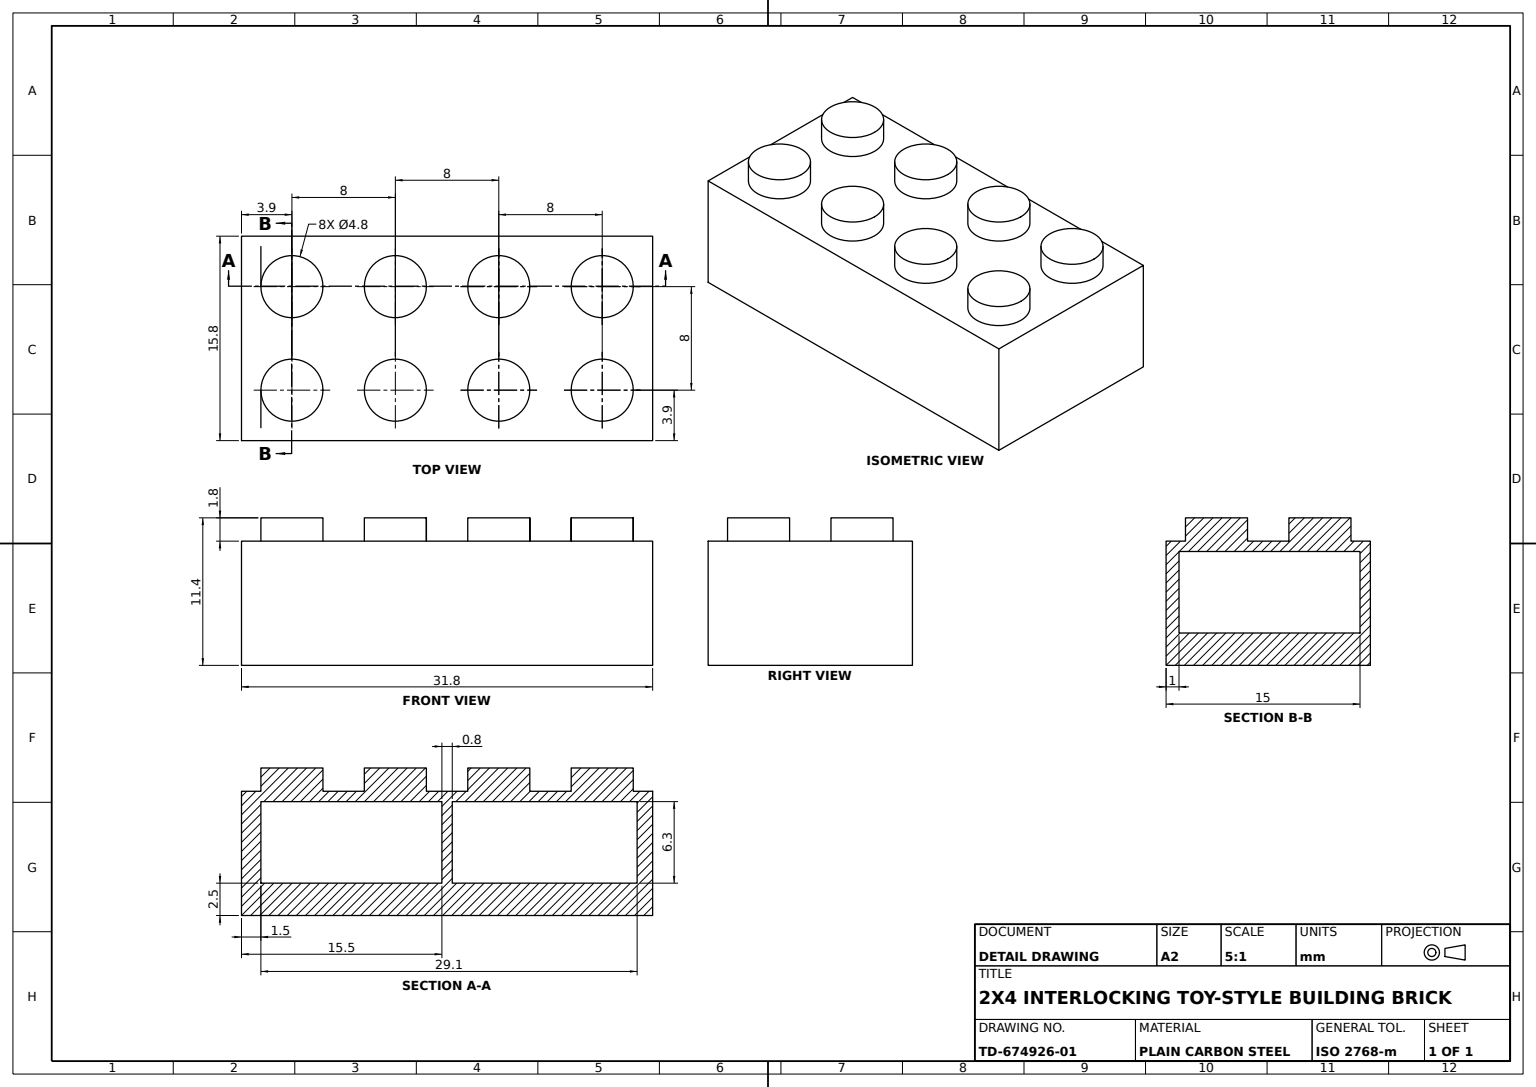
from build123d import *

# Parameters (mm, degrees)
BRICK_OUTLINE_SKETCH_W    = 31.8
BRICK_OUTLINE_SKETCH_H    = 15.8
BRICK_BODY_9_6_DEPTH      = 9.6
STUD_CIRCLES_SKETCH_R     = 2.4
STUDS_8X_4_8_DEPTH        = 1.8
UNDERSIDE_CUT_SKETCH_W    = 14
UNDERSIDE_CUT_SKETCH_H    = 6.3
UNDERSIDE_CUT_SKETCH_W_2  = 14.3
UNDERSIDE_CUT_DEPTH       = 15
UNDERSIDE_BOSS_SKETCH_W   = 14
UNDERSIDE_BOSS_SKETCH_H   = 6.3
UNDERSIDE_BOSS_SKETCH_W_2 = 14.3
UNDERSIDE_BOSS_1MM_DEPTH  = 1


with BuildPart() as part:
    # Brick Outline Sketch → Brick Body 9.6 (new body)
    with BuildSketch(Plane.XY):
        with Locations((15.9, 7.9)):
            Rectangle(BRICK_OUTLINE_SKETCH_W, BRICK_OUTLINE_SKETCH_H)
    extrude(amount=BRICK_BODY_9_6_DEPTH)

    # Stud Circles Sketch → Studs 8xØ4.8 (add)
    with BuildSketch(Plane.XY.offset(9.6)):
        with Locations(Location((3.9, 11.9, 0), (0, 0, 180))):
            Circle(STUD_CIRCLES_SKETCH_R)
        with Locations(Location((3.9, 3.9, 0), (0, 0, 180))):
            Circle(STUD_CIRCLES_SKETCH_R)
        with Locations(Location((11.9, 11.9, 0), (0, 0, 180))):
            Circle(STUD_CIRCLES_SKETCH_R)
        with Locations(Location((19.9, 11.9, 0), (0, 0, 180))):
            Circle(STUD_CIRCLES_SKETCH_R)
        with Locations(Location((27.9, 11.9, 0), (0, 0, 180))):
            Circle(STUD_CIRCLES_SKETCH_R)
        with Locations(Location((11.9, 3.9, 0), (0, 0, 180))):
            Circle(STUD_CIRCLES_SKETCH_R)
        with Locations(Location((19.9, 3.9, 0), (0, 0, 180))):
            Circle(STUD_CIRCLES_SKETCH_R)
        with Locations(Location((27.9, 3.9, 0), (0, 0, 180))):
            Circle(STUD_CIRCLES_SKETCH_R)
    extrude(amount=STUDS_8X_4_8_DEPTH)

    # Underside Cut Sketch → Underside Cut (cut)
    with BuildSketch(Plane.XZ):
        with Locations((8.5, 5.65)):
            Rectangle(UNDERSIDE_CUT_SKETCH_W, UNDERSIDE_CUT_SKETCH_H)
        with Locations((23.45, 5.65)):
            Rectangle(UNDERSIDE_CUT_SKETCH_W_2, UNDERSIDE_CUT_SKETCH_H)
    extrude(amount=-UNDERSIDE_CUT_DEPTH, mode=Mode.SUBTRACT)

    # Underside Boss Sketch → Underside Boss 1mm (add)
    with BuildSketch(Plane.XZ):
        with Locations((8.5, 5.65)):
            Rectangle(UNDERSIDE_BOSS_SKETCH_W, UNDERSIDE_BOSS_SKETCH_H)
        with Locations((23.45, 5.65)):
            Rectangle(UNDERSIDE_BOSS_SKETCH_W_2, UNDERSIDE_BOSS_SKETCH_H)
    extrude(amount=-UNDERSIDE_BOSS_1MM_DEPTH)


solid = part.part
